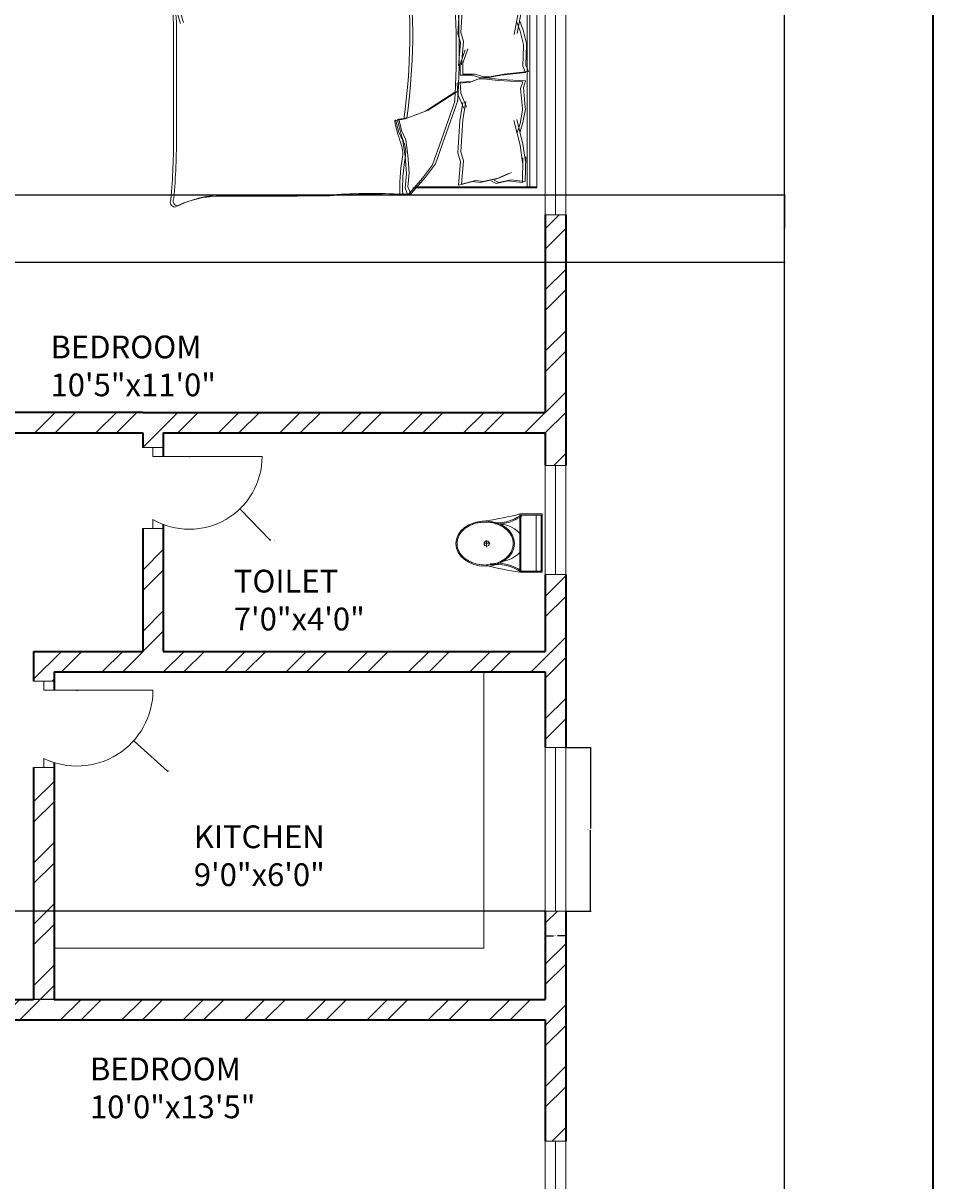
# Model space of a CAD drawing. Units: inches. Extents: x 2008 to 2657, y 1077 to 2165.
# Tile 7 of 16: x 2457 to 2657, y 1312 to 1567. Entities that reach past the tile are written whole.
import ezdxf

# ---------------------------------------------------------------- set-up
doc = ezdxf.new("R2010")
doc.units = ezdxf.units.IN
for name, color, linetype, lineweight in [('A-ANNO-DIMS', 2, 'Continuous', 18), ('A-ANNO-TTLB', 7, 'Continuous', 35), ('A-AREA-IDEN', 4, 'Continuous', 18), ('A-DOOR', 11, 'Continuous', 18), ('A-FLOR-CASE', 9, 'Continuous', 18), ('A-FLOR-FIXT', 8, 'Continuous', 18), ('A-FURN', 8, 'Continuous', 13), ('A-GLAZ', 191, 'Continuous', 18), ('A-WALL', 7, 'Continuous', 35)]:
    doc.layers.add(name, color=color, linetype=linetype, lineweight=lineweight)
doc.layers.add('A-WALL-PATT', color=30, linetype='Continuous', lineweight=13, true_color=0xf8991e)
doc.styles.get("Standard").update_dxf_attribs({"font": 'arial.ttf'})
doc.dimstyles.get("Standard").update_dxf_attribs({"dimtxt": 0.18, "dimasz": 0.18, "dimexe": 0.18, "dimexo": 0.0625, "dimgap": 0.09, "dimtad": 0, "dimtih": 1, "dimtoh": 1, "dimdec": 4, "dimzin": 0, "dimdsep": 46, "dimtxsty": 'Standard', "dimcen": 0.09, "dimadec": 0, "dimazin": 0, "dimtfac": 1, "dimtdec": 4, "dimtofl": 0, "dimtmove": 0, "dimatfit": 3, "dimfxl": 1, "dimtolj": 1, "dimtzin": 0, "dimarcsym": 0})

# ---------------------------------------------------------------- blocks, each defined once
blk = doc.blocks.new('A$C31115884')
for p, q in [((258, 466), (258, 523)), ((283, 498), (223, 498)), ((0, 200), (0, 0)), ((520, 200), (0, 200)), ((10, 190), (10, 10)), ((510, 190), (10, 190)), ((510, 10), (510, 190)), ((520, 0), (520, 200)), ((510, 54), (0, 54)), ((10, 10), (510, 10)), ((0, 0), (520, 0))]:
    blk.add_line(p, q)
blk.add_circle((256, 496), 23.6)
for centre, radius, start, end in [((2778, -205), 2807, 165.4549, 171.7133), ((-295, 403), 365, 324.2091, 9.3499), ((-295, 403), 375, 324.2091, 9.3499), ((139, 406), 293, 315.8436, 2.6563), ((806, 403), 365, 170.6501, 215.7909), ((3237, 905), 2807, 188.2867, 194.5451), ((384, 406), 293, 190.2774, 224.1564), ((806, 403), 375, 179.2036, 215.7909)]:
    blk.add_arc(centre, radius, start, end)
blk.add_ellipse((256, 510), major_axis=(0, -261), ratio=0.772727)
blk.add_open_spline([(256, 259), (263, 259), (270, 260), (288, 262), (299, 265), (320, 273), (330, 278), (350, 291), (360, 299), (378, 316), (386, 326), (402, 347), (409, 358), (421, 383), (427, 395), (436, 422), (440, 436), (445, 465), (447, 480), (448, 509), (448, 524), (445, 553), (443, 568), (436, 596), (432, 610), (422, 636), (416, 649), (402, 672), (395, 683), (379, 703), (370, 712), (351, 728), (341, 735), (321, 746), (310, 751), (289, 757), (278, 759), (256, 761), (245, 761), (223, 757), (212, 754), (191, 746), (181, 741), (161, 728), (151, 720), (133, 703), (125, 693), (110, 672), (103, 660), (90, 636), (85, 623), (76, 596), (72, 582), (67, 553), (66, 538), (64, 509), (65, 494), (68, 465), (70, 450), (77, 422), (81, 408), (91, 382), (97, 370), (111, 346), (118, 335), (135, 316), (144, 307), (162, 291), (172, 284), (193, 273), (203, 269), (225, 262), (236, 260), (250, 259), (253, 259), (256, 259)], degree=3, knots=[0, 0, 0, 0, 0.110105, 0.110105, 0.285049, 0.285049, 0.459994, 0.459994, 0.634938, 0.634938, 0.809882, 0.809882, 0.984827, 0.984827, 1.159771, 1.159771, 1.334715, 1.334715, 1.50966, 1.50966, 1.684604, 1.684604, 1.859549, 1.859549, 2.034493, 2.034493, 2.209437, 2.209437, 2.384382, 2.384382, 2.559326, 2.559326, 2.73427, 2.73427, 2.909215, 2.909215, 3.084159, 3.084159, 3.259103, 3.259103, 3.434048, 3.434048, 3.608992, 3.608992, 3.783936, 3.783936, 3.958881, 3.958881, 4.133825, 4.133825, 4.30877, 4.30877, 4.483714, 4.483714, 4.658658, 4.658658, 4.833603, 4.833603, 5.008547, 5.008547, 5.183491, 5.183491, 5.358436, 5.358436, 5.53338, 5.53338, 5.708324, 5.708324, 5.883269, 5.883269, 6.058213, 6.058213, 6.233158, 6.233158, 6.283185, 6.283185, 6.283185, 6.283185])
blk = doc.blocks.new('BED-DOUBLE')
for p, q in [((0, 51.49), (0.64, 51.49)), ((0, 3.48), (0, 51.49)), ((0, 51.27), (26.61, 51.27)), ((0, 51.27), (26.61, 51.27)), ((0.64, 51.49), (27.25, 51.49)), ((0.64, 51.49), (27.25, 51.49)), ((1.53, 3.48), (1.53, 51.27)), ((1.53, 3.48), (1.53, 51.27)), ((2.17, 3.7), (2.17, 51.49)), ((2.17, 3.7), (2.17, 51.49)), ((17.21, 50.93), (14.07, 50.15)), ((17.21, 50.93), (14.07, 50.15)), ((16.81, 45.8), (17.21, 50.93)), ((16.81, 45.8), (17.21, 50.93)), ((27.75, 52.87), (24.5, 49.16)), ((27.75, 52.87), (24.5, 49.16)), ((28.39, 53.1), (25.14, 49.39)), ((28.39, 53.1), (25.14, 49.39)), ((29.49, 52.95), (27.75, 52.87, 3.87)), ((29.49, 52.95), (27.75, 52.87, 3.87)), ((28.37, 51.33), (27.75, 52.87)), ((28.37, 51.33), (27.75, 52.87)), ((28.06, 48.23), (28.37, 51.33)), ((28.06, 48.23), (28.37, 51.33)), ((30.13, 53.18), (28.39, 53.1, 3.87)), ((30.13, 53.18), (28.39, 53.1, 3.87)), ((29, 51.56), (28.39, 53.1)), ((29, 51.56), (28.39, 53.1)), ((28.7, 48.46), (29, 51.56)), ((28.7, 48.46), (29, 51.56)), ((2.56, 50.11), (2.46, 44.71)), ((2.56, 50.11), (2.46, 44.71)), ((2.56, 50.11), (5.77, 49.73)), ((2.56, 50.11), (5.77, 49.73)), ((3.2, 50.34), (3.1, 44.94)), ((3.2, 50.34), (3.1, 44.94)), ((3.2, 50.34), (6.41, 49.96)), ((3.2, 50.34), (6.41, 49.96)), ((8.26, 49.31), (5.58, 48.13)), ((8.26, 49.31), (5.58, 48.13)), ((5.77, 49.73), (8.34, 50.33)), ((5.77, 49.73), (8.34, 50.33)), ((8.9, 49.54), (6.22, 48.36)), ((8.9, 49.54), (6.22, 48.36)), ((6.41, 49.96), (8.98, 50.56)), ((6.41, 49.96), (8.98, 50.56)), ((11.83, 50.11), (8.26, 49.31)), ((11.83, 50.11), (8.26, 49.31)), ((8.34, 50.33), (9.38, 49.82)), ((8.34, 50.33), (9.38, 49.81)), ((12.47, 50.34), (8.9, 49.54)), ((12.47, 50.34), (8.9, 49.54)), ((8.98, 50.56), (10.02, 50.04)), ((8.98, 50.56), (10.02, 50.04)), ((13.43, 49.92), (11.83, 50.11)), ((13.43, 49.92), (11.83, 50.11)), ((14.07, 50.15), (12.47, 50.34)), ((14.07, 50.15), (12.47, 50.34)), ((16.57, 50.7), (13.43, 49.92)), ((16.57, 50.7), (13.43, 49.92)), ((16.17, 45.57), (16.57, 50.7)), ((16.17, 45.57), (16.57, 50.7)), ((24.5, 49.16), (22.33, 46.22)), ((24.5, 49.16), (22.33, 46.22)), ((25.14, 49.39), (22.97, 46.45)), ((25.14, 49.39), (22.97, 46.45)), ((29, 44.59), (28.7, 48.46)), ((29, 44.59), (28.7, 48.46)), ((3.1, 44.94), (3.18, 45.94)), ((3.1, 44.94), (3.18, 45.94)), ((3.18, 45.94), (3.71, 42.14)), ((3.18, 45.94), (3.71, 42.14)), ((22.33, 46.22), (20.32, 40.64)), ((22.33, 46.22), (20.32, 40.64)), ((22.97, 46.45), (20.96, 40.87)), ((22.97, 46.45), (20.96, 40.87)), ((28.37, 44.36), (28.06, 48.23)), ((28.37, 44.36), (28.06, 48.23)), ((2.46, 44.71), (2.54, 45.71)), ((2.46, 44.71), (2.54, 45.71)), ((2.54, 45.71), (3.07, 41.91)), ((2.54, 45.71), (3.07, 41.91)), ((16.73, 43.61), (16.17, 45.57)), ((16.73, 43.61), (16.17, 45.57)), ((16.3, 36.6), (16.73, 43.61)), ((16.3, 36.6), (16.73, 43.61)), ((17.37, 43.84), (16.81, 45.8)), ((17.37, 43.83), (16.81, 45.8)), ((16.93, 36.83), (17.37, 43.84)), ((16.93, 36.82), (17.37, 43.83)), ((28.83, 40.95), (28.37, 44.36)), ((28.83, 40.95), (28.37, 44.36)), ((29.47, 41.18), (29, 44.59)), ((29.47, 41.18), (29, 44.59)), ((3.07, 41.91), (4.42, 36.5)), ((3.07, 41.91), (4.42, 36.5)), ((3.71, 42.14), (5.06, 36.72)), ((3.71, 42.14), (5.06, 36.72)), ((20.96, 40.87), (18.02, 32.54)), ((20.96, 40.87), (18.02, 32.53)), ((29.76, 38.94), (28.83, 40.95)), ((29.76, 38.94), (28.83, 40.95)), ((30.4, 39.17), (29.47, 41.18)), ((30.4, 39.17), (29.47, 41.18)), ((3.67, 39.2), (3.08, 37.14)), ((3.67, 39.2), (3.08, 37.14)), ((4.31, 39.43), (3.72, 37.36)), ((4.31, 39.43), (3.72, 37.36)), ((20.32, 40.64), (17.38, 32.31)), ((20.32, 40.64), (17.38, 32.31)), ((30.38, 36.46), (29.76, 38.94)), ((30.38, 36.46), (29.76, 38.94)), ((31.02, 36.69), (30.4, 39.17)), ((31.02, 36.69), (30.4, 39.17)), ((79.25, 15.06), (79.25, 39.68)), ((79.25, 15.06), (79.25, 39.68)), ((79.88, 15.29), (79.88, 39.91)), ((79.88, 15.29), (79.88, 39.91)), ((3.08, 37.14), (2.54, 34.21)), ((3.08, 37.14), (2.54, 34.2)), ((3.72, 37.36), (3.18, 34.43)), ((3.72, 37.36), (3.18, 34.43)), ((15.63, 32.56), (16.3, 36.6)), ((15.63, 32.56), (16.3, 36.6)), ((16.27, 32.79), (16.93, 36.83)), ((16.27, 32.79), (16.93, 36.82)), ((23.88, 34.45), (28.37, 36.15)), ((23.88, 34.45), (28.37, 36.15)), ((24.52, 34.68), (29, 36.38)), ((24.52, 34.68), (29, 36.38)), ((28.37, 36.15), (30.38, 36.46)), ((28.37, 36.15), (30.38, 36.46)), ((29, 36.38), (31.02, 36.69)), ((29, 36.38), (31.02, 36.69)), ((2.54, 34.21), (2.56, 33.88)), ((2.54, 34.2), (2.56, 33.88)), ((2.56, 33.88), (2.98, 29.46)), ((2.56, 33.88), (2.98, 29.46)), ((3.18, 34.43), (3.2, 34.11)), ((3.18, 34.43), (3.2, 34.11)), ((3.2, 34.11), (3.62, 29.68)), ((3.2, 34.11), (3.62, 29.68)), ((16.74, 30.75), (15.45, 33.82)), ((16.74, 30.75), (15.45, 33.82)), ((17.38, 30.98), (16.09, 34.05)), ((17.38, 30.98), (16.09, 34.05)), ((17.38, 30.26), (23.88, 34.45)), ((17.38, 30.26), (23.88, 34.45)), ((18.02, 30.49), (24.52, 34.68)), ((18.02, 30.49), (24.52, 34.68)), ((16.89, 28.3), (16.74, 30.75)), ((16.89, 28.3), (16.74, 30.75)), ((17.53, 28.53), (17.38, 30.98)), ((17.53, 28.53), (17.38, 30.98)), ((2.98, 29.46), (2.49, 27.98)), ((2.98, 29.46), (2.49, 27.98)), ((3.62, 29.68), (3.13, 28.21)), ((3.62, 29.68), (3.13, 28.21)), ((3.13, 28.21), (8.51, 27.96)), ((3.13, 28.21), (8.51, 27.96)), ((12.38, 27.44), (14.22, 28.13)), ((12.38, 27.44), (14.22, 28.13)), ((13.02, 27.66), (14.86, 28.36)), ((13.02, 27.66), (14.86, 28.36)), ((14.22, 28.13), (16.89, 28.3)), ((14.22, 28.13), (16.89, 28.3)), ((14.86, 28.36), (17.53, 28.53)), ((14.86, 28.36), (17.53, 28.53)), ((1.87, 25.98), (7.22, 26.56)), ((1.87, 25.98), (7.22, 26.56)), ((2.45, 24.54), (1.87, 25.98)), ((2.45, 24.54), (1.87, 25.98)), ((2.49, 27.98), (7.87, 27.73)), ((2.49, 27.98), (7.87, 27.73)), ((2.51, 26.21), (7.86, 26.79)), ((2.51, 26.21), (7.86, 26.79)), ((3.09, 24.77), (2.51, 26.21)), ((3.09, 24.77), (2.51, 26.21)), ((7.22, 26.56), (10.4, 27.14)), ((7.22, 26.56), (10.4, 27.14)), ((7.86, 26.79), (11.04, 27.37)), ((7.86, 26.79), (11.04, 27.37)), ((7.87, 27.73), (11.08, 27.36)), ((7.87, 27.73), (11.08, 27.36)), ((8.51, 27.96), (11.72, 27.58)), ((8.51, 27.96), (11.72, 27.58)), ((10.4, 27.14), (11.7, 27.14)), ((10.4, 27.14), (11.7, 27.14)), ((11.04, 27.37), (12.34, 27.37)), ((11.04, 27.37), (12.34, 27.37)), ((11.08, 27.36), (12.38, 27.44)), ((11.08, 27.36), (12.38, 27.44)), ((11.7, 27.14), (13.58, 26.56)), ((11.7, 27.14), (13.58, 26.56)), ((11.72, 27.58), (13.02, 27.66)), ((11.72, 27.58), (13.02, 27.66)), ((12.34, 27.37), (14.22, 26.79)), ((12.34, 27.37), (14.22, 26.79)), ((13.58, 26.56), (16.26, 26.56)), ((13.58, 26.56), (16.26, 26.56)), ((14.22, 26.79), (16.9, 26.79)), ((14.22, 26.79), (16.9, 26.79)), ((16.26, 26.56), (16.26, 24.1)), ((16.26, 26.56), (16.26, 24.1)), ((16.9, 26.79), (16.9, 24.33)), ((16.9, 26.79), (16.9, 24.33)), ((2.3, 20.09), (2.45, 24.54)), ((2.3, 20.09), (2.45, 24.54)), ((2.94, 20.32), (3.09, 24.77)), ((2.94, 20.32), (3.09, 24.77)), ((16.26, 24.1), (15.17, 20.96)), ((16.26, 24.1), (15.17, 20.96)), ((16.9, 24.33), (15.81, 21.19)), ((16.9, 24.33), (15.81, 21.19)), ((16.17, 19.38), (16.57, 24.52)), ((16.17, 19.38), (16.57, 24.52)), ((16.81, 19.61), (17.21, 24.74)), ((16.81, 19.61), (17.21, 24.74)), ((2.3, 19.77), (2.3, 20.09)), ((2.3, 19.77), (2.3, 20.09)), ((3.03, 16.88), (2.3, 19.77)), ((3.03, 16.88), (2.3, 19.77)), ((2.94, 20), (2.94, 20.32)), ((2.94, 20), (2.94, 20.32)), ((3.67, 17.11), (2.94, 20)), ((3.67, 17.11), (2.94, 20)), ((3.96, 12.34), (4.97, 17.83)), ((3.96, 12.34), (4.97, 17.83)), ((16.73, 17.42), (16.17, 19.38)), ((16.73, 17.42), (16.17, 19.38)), ((17.37, 17.65), (16.81, 19.61)), ((17.37, 17.65), (16.81, 19.61)), ((3.75, 14.86), (3.03, 16.88)), ((3.75, 14.86), (3.03, 16.88)), ((3.32, 12.11), (4.33, 17.6)), ((3.32, 12.11), (4.33, 17.6)), ((4.39, 15.08), (3.67, 17.11)), ((4.39, 15.08), (3.67, 17.11)), ((16.3, 10.41), (16.73, 17.42)), ((16.3, 10.41), (16.73, 17.42)), ((16.93, 10.64), (17.37, 17.65)), ((16.93, 10.64), (17.37, 17.65)), ((3.03, 8.29), (3.32, 12.11)), ((3.03, 8.29), (3.32, 12.11)), ((3.67, 8.51), (3.96, 12.34)), ((3.67, 8.51), (3.96, 12.34)), ((15.63, 6.38), (16.3, 10.41)), ((15.63, 6.38), (16.3, 10.41)), ((16.27, 6.61), (16.93, 10.64)), ((16.27, 6.61), (16.93, 10.64)), ((16.3, 10.41), (16.62, 9.28)), ((16.3, 10.41), (16.62, 9.28)), ((16.93, 10.64), (17.26, 9.51)), ((16.93, 10.64), (17.26, 9.51)), ((3.01, 8.18), (3.03, 8.29)), ((3.01, 8.18), (3.03, 8.29)), ((3.34, 3.9), (3.01, 8.18)), ((3.34, 3.9), (3.01, 8.18)), ((3.65, 8.41), (3.67, 8.51)), ((3.65, 8.41), (3.67, 8.51)), ((3.98, 4.13), (3.65, 8.41)), ((3.98, 4.13), (3.65, 8.41)), ((16.62, 9.28), (17.34, 4.18)), ((16.62, 9.28), (17.34, 4.18)), ((17.26, 9.51), (17.98, 4.41)), ((17.26, 9.51), (17.98, 4.41)), ((8.96, 5.05), (6.21, 6.06)), ((8.96, 5.05), (6.21, 6.06)), ((9.59, 5.28), (6.85, 6.29)), ((9.59, 5.28), (6.85, 6.29)), ((13.21, 4.7), (9.59, 5.28)), ((13.21, 4.7), (9.59, 5.28)), ((18.11, 3.48), (0, 3.48)), ((18.11, 3.48), (0, 3.48)), ((18.75, 3.7), (0.64, 3.7)), ((18.75, 3.7), (0.64, 3.7)), ((3.32, 3.9), (6.5, 4.47)), ((3.32, 3.89), (6.5, 4.47)), ((3.96, 4.12), (7.14, 4.7)), ((3.96, 4.12), (7.14, 4.7)), ((6.5, 4.47), (9.1, 4.04)), ((6.5, 4.47), (9.1, 4.04)), ((7.14, 4.7), (9.74, 4.27)), ((7.14, 4.7), (9.74, 4.27)), ((12.57, 4.47), (8.96, 5.05)), ((12.57, 4.47), (8.96, 5.05)), ((9.1, 4.04), (10.11, 4.62)), ((9.1, 4.04), (10.11, 4.62)), ((9.74, 4.27), (10.75, 4.85)), ((9.74, 4.27), (10.75, 4.85)), ((14.16, 4.76), (12.57, 4.47)), ((14.16, 4.76), (12.57, 4.47)), ((14.8, 4.99), (13.21, 4.7)), ((14.8, 4.99), (13.21, 4.7)), ((17.34, 4.18), (14.16, 4.76)), ((17.34, 4.18), (14.16, 4.76)), ((17.98, 4.41), (14.8, 4.99)), ((17.98, 4.41), (14.8, 4.99))]:
    blk.add_line(p, q)
for centre, radius, start, end in [((68.67, 76.16), 23.07, 267.4714, 296.4681), ((68.67, 76.16), 23.07, 267.4714, 296.4681), ((69.31, 76.39), 23.07, 267.4714, 296.4681), ((69.31, 76.39), 23.07, 267.4714, 296.4681), ((78.87, 54.41), 1.1, 332.6588, 86.02), ((78.87, 54.41), 1.1, 332.6588, 86.02), ((212.28, 41.15), 133.04, 174.4998, 180.6351), ((212.28, 41.15), 133.04, 174.4998, 180.6351), ((79.51, 54.64), 1.1, 332.6588, 86.02), ((79.51, 54.64), 1.1, 332.6588, 86.02), ((212.92, 41.38), 133.04, 174.4998, 180.6351), ((212.92, 41.38), 133.04, 174.4998, 180.6351), ((-6.66, 51.33), 36.18, 349.8763, 2.5657), ((-6.66, 51.33), 36.18, 349.8763, 2.5657), ((36.32, 182.27), 129.5, 266.9791, 273.8365), ((36.32, 182.27), 129.5, 266.9791, 273.8365), ((-6.02, 51.56), 36.18, 349.8763, 2.5657), ((-6.02, 51.56), 36.18, 349.8763, 2.5657), ((36.95, 182.49), 129.5, 266.9791, 273.8365), ((36.95, 182.49), 129.5, 266.9791, 273.8365), ((67.82, -4508.74), 4561.86, 90.00217, 90.28689), ((67.82, -4508.74), 4561.86, 90.00217, 90.28689), ((68.46, -4508.51), 4561.86, 90.00217, 90.28689), ((68.46, -4508.51), 4561.86, 90.00217, 90.28689), ((35.07, 43.74), 6.22, 168.6608, 203.7384), ((35.07, 43.74), 6.22, 168.6608, 203.7384), ((35.71, 43.97), 6.22, 168.6608, 203.7384), ((35.71, 43.97), 6.22, 168.6608, 203.7384), ((1.48, 31.15), 29.65, 10.6617, 19.8806), ((1.48, 31.15), 29.65, 10.6617, 19.8806), ((2.12, 31.38), 29.65, 10.6617, 19.8806), ((2.12, 31.38), 29.65, 10.6617, 19.8806), ((156.32, 17.76), 129.02, 171.7845, 186.9006), ((156.32, 17.76), 129.02, 171.7845, 186.9006), ((156.96, 17.98), 129.02, 171.7845, 186.9006), ((156.96, 17.98), 129.02, 171.7845, 186.9006), ((30.44, 36.64), 0.185, 250.2464, 1.1377), ((30.44, 36.64), 0.185, 250.2464, 1.1377), ((31.08, 36.87), 0.185, 250.2464, 1.1377), ((31.08, 36.86), 0.185, 250.2464, 1.1377), ((182.05, 21.36), 164.97, 176.0865, 186.7821), ((182.05, 21.36), 164.97, 176.0865, 186.7821), ((182.69, 21.59), 164.97, 176.0865, 186.7821), ((182.69, 21.59), 164.97, 176.0865, 186.7821), ((-23.07, -16.99), 106.46, 13.3832, 17.7053), ((-23.07, -16.99), 106.46, 13.3832, 17.7053), ((201.48, 21.66), 121.76, 182.9958, 189.4091), ((201.48, 21.66), 121.76, 182.9958, 189.4091), ((-23.71, -17.22), 106.46, 13.3832, 17.7053), ((-23.71, -17.22), 106.46, 13.3832, 17.7053), ((200.84, 21.43), 121.76, 182.9958, 189.4091), ((200.84, 21.43), 121.76, 182.9958, 189.4091), ((31.17, -167.31), 170.11, 88.4762, 91.0082), ((31.17, -167.31), 170.11, 88.4762, 91.0082), ((31.81, -167.08), 170.11, 88.4762, 91.0082), ((31.81, -167.08), 170.11, 88.4762, 91.0082), ((50.61, 484.82), 482.31, 268.2277, 271.7185), ((50.61, 484.82), 482.31, 268.2277, 271.7185), ((51.25, 485.05), 482.31, 268.2277, 271.7185), ((51.25, 485.05), 482.31, 268.2277, 271.7185), ((64.52, -26.9), 29.63, 76.0648, 88.9113), ((64.52, -26.9), 29.63, 76.0648, 88.9113), ((65.15, -26.67), 29.63, 76.0648, 88.9113), ((65.15, -26.67), 29.63, 76.0648, 88.9113), ((20.1, 85.16), 83.31, 268.7218, 275.604), ((20.1, 85.16), 83.31, 268.7218, 275.604), ((20.74, 85.39), 83.31, 268.7218, 275.604), ((20.74, 85.39), 83.31, 268.7218, 275.604), ((70.28, -21.66), 23.56, 67.9751, 86.652), ((70.28, -21.66), 23.56, 67.9751, 86.652), ((70.92, -21.43), 23.56, 67.9751, 86.652), ((70.92, -21.43), 23.56, 67.9751, 86.652), ((79.72, 1.09), 1.09, 236.1736, 23.4781), ((79.72, 1.09), 1.09, 236.1736, 23.4781), ((80.36, 1.32), 1.09, 236.1736, 23.4781), ((80.36, 1.32), 1.09, 236.1736, 23.4781)]:
    blk.add_arc(centre, radius, start, end)
blk = doc.blocks.new('WIN-60IN-B')
for p, q in [((0, 4.5), (0, 0)), ((0, 4.5), (60, 4.5)), ((60, 2.25), (60, 4.5)), ((60, 4.5), (60, 0)), ((0, 0), (0, 2.25)), ((0, 2.25), (60, 2.25)), ((60, 0), (0, 0))]:
    blk.add_line(p, q)
blk = doc.blocks.new('WIN-24IN-B')
for p, q in [((0, 24), (4.5, 24)), ((0, 24), (0, 0)), ((4.5, 24), (2.25, 24)), ((2.25, 24), (2.25, 0)), ((4.5, 0), (4.5, 24)), ((2.25, 0), (0, 0)), ((0, 0), (4.5, 0))]:
    blk.add_line(p, q)
blk = doc.blocks.new('WIN-36IN-A')
for p, q in [((0, 36), (4.5, 36)), ((0, 0), (0, 36)), ((4.5, 36), (2.25, 36)), ((2.25, 36), (2.25, 0)), ((4.5, 36), (4.5, 0)), ((4.5, 0), (0, 0)), ((2.25, 0), (4.5, 0))]:
    blk.add_line(p, q)
blk = doc.blocks.new('*D27')
at = {"layer": 'A-ANNO-DIMS', "color": 0, "lineweight": -2, "transparency": 16777216}
for p, q in [((2576.82, 1407.57), (2582.34, 1407.57)), ((2582.16, 1407.39), (2582.16, 1389.75)), ((2582.16, 1371.75), (2582.16, 1389.39)), ((2576.82, 1371.57), (2582.34, 1371.57))]:
    blk.add_line(p, q, dxfattribs=at)
at = {"layer": 'A-ANNO-DIMS', "color": 0, "transparency": 16777216}
for points in [[(2582.13, 1407.39), (2582.19, 1407.39), (2582.16, 1407.57)], [(2582.13, 1371.75), (2582.19, 1371.75), (2582.16, 1371.57)]]:
    blk.add_solid(points, dxfattribs=at)
at = {"layer": 'Defpoints', "color": 0, "transparency": 16777216}
for p in [(2576.76, 1407.57), (2582.16, 1407.57), (2576.76, 1371.57)]:
    blk.add_point(p, dxfattribs=at)
at = {"layer": 'A-ANNO-DIMS', "color": 0, "transparency": 16777216, "insert": (2582.16, 1389.57), "char_height": 0.18, "attachment_point": 5}
blk.add_mtext('\\A1;WIN A 36 TYP.', dxfattribs=at)
blk = doc.blocks.new('*D28')
at = {"layer": 'A-ANNO-DIMS', "color": 0, "lineweight": -2, "transparency": 16777216}
for p, q in [((2572.26, 1371.51), (2572.26, 1365.99)), ((2576.76, 1371.51), (2576.76, 1365.99)), ((2572.44, 1366.17), (2574.05, 1366.17)), ((2576.58, 1366.17), (2574.97, 1366.17))]:
    blk.add_line(p, q, dxfattribs=at)
at = {"layer": 'A-ANNO-DIMS', "color": 0, "transparency": 16777216}
for points in [[(2572.44, 1366.2), (2572.44, 1366.14), (2572.26, 1366.17)], [(2576.58, 1366.2), (2576.58, 1366.14), (2576.76, 1366.17)]]:
    blk.add_solid(points, dxfattribs=at)
at = {"layer": 'Defpoints', "color": 0, "transparency": 16777216}
for p in [(2572.26, 1371.57), (2576.76, 1371.57), (2576.76, 1366.17)]:
    blk.add_point(p, dxfattribs=at)
at = {"layer": 'A-ANNO-DIMS', "color": 0, "transparency": 16777216, "insert": (2574.51, 1366.17), "char_height": 0.18, "attachment_point": 5}
blk.add_mtext('\\A1;5 TYP.', dxfattribs=at)
blk = doc.blocks.new('*D31')
at = {"layer": 'A-ANNO-DIMS', "color": 0, "lineweight": -2, "transparency": 16777216}
for p, q in [((2076.26, 1562.18), (2076.26, 1140.44)), ((2576.76, 1188.61), (2576.76, 1140.44)), ((2076.44, 1140.62), (2326.12, 1140.62)), ((2576.58, 1140.62), (2326.91, 1140.62))]:
    blk.add_line(p, q, dxfattribs=at)
at = {"layer": 'A-ANNO-DIMS', "color": 0, "transparency": 16777216}
for points in [[(2076.44, 1140.65), (2076.44, 1140.59), (2076.26, 1140.62)], [(2576.58, 1140.65), (2576.58, 1140.59), (2576.76, 1140.62)]]:
    blk.add_solid(points, dxfattribs=at)
at = {"layer": 'Defpoints', "color": 0, "transparency": 16777216}
for p in [(2076.26, 1562.24), (2576.76, 1188.67), (2576.76, 1140.62)]:
    blk.add_point(p, dxfattribs=at)
at = {"layer": 'A-ANNO-DIMS', "color": 0, "transparency": 16777216, "insert": (2326.51, 1140.62), "char_height": 0.18, "attachment_point": 5}
blk.add_mtext('\\A1;500.5', dxfattribs=at)
blk = doc.blocks.new('*D32')
at = {"layer": 'A-ANNO-DIMS', "color": 0, "lineweight": -2, "transparency": 16777216}
for p, q in [((2576.82, 2094.67), (2624.99, 2094.67)), ((2624.81, 2094.49), (2624.81, 1641.86)), ((2624.81, 1188.85), (2624.81, 1641.49)), ((2576.82, 1188.67), (2624.99, 1188.67))]:
    blk.add_line(p, q, dxfattribs=at)
at = {"layer": 'A-ANNO-DIMS', "color": 0, "transparency": 16777216}
for points in [[(2624.78, 2094.49), (2624.84, 2094.49), (2624.81, 2094.67)], [(2624.78, 1188.85), (2624.84, 1188.85), (2624.81, 1188.67)]]:
    blk.add_solid(points, dxfattribs=at)
at = {"layer": 'Defpoints', "color": 0, "transparency": 16777216}
for p in [(2576.76, 2094.67), (2624.81, 2094.67), (2576.76, 1188.67)]:
    blk.add_point(p, dxfattribs=at)
at = {"layer": 'A-ANNO-DIMS', "color": 0, "transparency": 16777216, "insert": (2624.81, 1641.67), "char_height": 0.18, "attachment_point": 5}
blk.add_mtext('\\A1;906', dxfattribs=at)
blk = doc.blocks.new('*D68')
at = {"layer": 'A-ANNO-DIMS', "color": 0, "lineweight": -2, "transparency": 16777216}
for p, q in [((2572.2, 1371.57), (2028.03, 1371.57)), ((2028.21, 1371.39), (2028.21, 1362.05)), ((2028.21, 1352.35), (2028.21, 1361.69)), ((2572.2, 1352.17), (2028.03, 1352.17))]:
    blk.add_line(p, q, dxfattribs=at)
at = {"layer": 'A-ANNO-DIMS', "color": 0, "transparency": 16777216}
for points in [[(2028.18, 1371.39), (2028.24, 1371.39), (2028.21, 1371.57)], [(2028.18, 1352.35), (2028.24, 1352.35), (2028.21, 1352.17)]]:
    blk.add_solid(points, dxfattribs=at)
at = {"layer": 'Defpoints', "color": 0, "transparency": 16777216}
for p in [(2028.21, 1371.57), (2572.26, 1371.57), (2572.26, 1352.17)]:
    blk.add_point(p, dxfattribs=at)
at = {"layer": 'A-ANNO-DIMS', "color": 0, "transparency": 16777216, "insert": (2028.21, 1361.87), "char_height": 0.18, "attachment_point": 5}
blk.add_mtext('\\A1;19.394', dxfattribs=at)
blk = doc.blocks.new('*D69')
at = {"layer": 'A-ANNO-DIMS', "color": 0, "lineweight": -2, "transparency": 16777216}
for p, q in [((2109.32, 1529), (2624.99, 1529)), ((2624.81, 1528.82), (2624.81, 1521.8)), ((2624.81, 1514.42), (2624.81, 1521.44)), ((2109.32, 1514.24), (2624.99, 1514.24))]:
    blk.add_line(p, q, dxfattribs=at)
at = {"layer": 'A-ANNO-DIMS', "color": 0, "transparency": 16777216}
for points in [[(2624.78, 1528.82), (2624.84, 1528.82), (2624.81, 1529)], [(2624.78, 1514.42), (2624.84, 1514.42), (2624.81, 1514.24)]]:
    blk.add_solid(points, dxfattribs=at)
at = {"layer": 'Defpoints', "color": 0, "transparency": 16777216}
for p in [(2109.26, 1529), (2624.81, 1529), (2109.26, 1514.24)]:
    blk.add_point(p, dxfattribs=at)
at = {"layer": 'A-ANNO-DIMS', "color": 0, "transparency": 16777216, "insert": (2624.81, 1521.62), "char_height": 0.18, "attachment_point": 5}
blk.add_mtext('\\A1;14.756', dxfattribs=at)
blk = doc.blocks.new('*D94')
at = {"layer": 'A-ANNO-DIMS', "color": 0, "lineweight": -2, "transparency": 16777216}
for p, q in [((2493.94, 1471.51), (2494.12, 1471.51)), ((2494.03, 1471.42), (2494.03, 1471.6)), ((2511.77, 1453.08), (2505.24, 1459.86)), ((2511.95, 1453.08), (2511.77, 1453.08))]:
    blk.add_line(p, q, dxfattribs=at)
at = {"layer": 'A-ANNO-DIMS', "color": 0, "transparency": 16777216}
blk.add_solid([(2505.26, 1459.88), (2505.22, 1459.84), (2505.12, 1459.99)], dxfattribs=at)
at = {"layer": 'Defpoints', "color": 0, "transparency": 16777216}
for p in [(2494.03, 1471.51), (2505.12, 1459.99)]:
    blk.add_point(p, dxfattribs=at)
at = {"layer": 'A-ANNO-DIMS', "color": 0, "transparency": 16777216, "insert": (2512.5, 1453.08), "char_height": 0.18, "attachment_point": 5}
blk.add_mtext('\\A1;R15.985', dxfattribs=at)
blk = doc.blocks.new('*D95')
at = {"layer": 'A-ANNO-DIMS', "color": 0, "lineweight": -2, "transparency": 16777216}
for p, q in [((2469.23, 1420.15), (2469.41, 1420.15)), ((2469.32, 1420.06), (2469.32, 1420.24)), ((2489.24, 1402.36), (2481.9, 1408.91)), ((2489.42, 1402.36), (2489.24, 1402.36))]:
    blk.add_line(p, q, dxfattribs=at)
at = {"layer": 'A-ANNO-DIMS', "color": 0, "transparency": 16777216}
blk.add_solid([(2481.92, 1408.93), (2481.88, 1408.89), (2481.77, 1409.03)], dxfattribs=at)
at = {"layer": 'Defpoints', "color": 0, "transparency": 16777216}
for p in [(2469.32, 1420.15), (2481.77, 1409.03)]:
    blk.add_point(p, dxfattribs=at)
at = {"layer": 'A-ANNO-DIMS', "color": 0, "transparency": 16777216, "insert": (2489.97, 1402.36), "char_height": 0.18, "attachment_point": 5}
blk.add_mtext('\\A1;R16.696', dxfattribs=at)

msp = doc.modelspace()

# ---------------------------------------------------------------- hatches: boundary and pattern name
at = {"layer": 'A-WALL-PATT'}
h = msp.add_hatch(dxfattribs=at)
h.set_pattern_fill('ANSI32', color=256)
h.paths.add_polyline_path([(2109.2619, 2094.6743), (2104.7619, 2094.6743), (2104.7619, 2072.1743), (2104.7619, 2021.6151), (2109.2619, 2021.6151), (2109.2619, 2055.6743), (2126.1387, 2055.6743), (2126.1387, 2057.9243), (2126.1387, 2060.1743), (2109.2619, 2060.1743)])
h.paths.add_polyline_path([(2223.2494, 2057.9243), (2223.2494, 2060.1743), (2186.1387, 2060.1743), (2186.1387, 2055.6743), (2223.2494, 2055.6743)])
h.paths.add_polyline_path([(2250.7619, 2072.1743), (2250.7619, 2090.1743), (2250.7619, 2094.6743), (2246.2619, 2094.6743), (2246.2619, 2060.1743), (2242.7242, 2060.1743), (2242.7242, 2055.6743), (2246.2619, 2055.6743), (2246.2619, 1899.6743), (2242.7458, 1899.6743), (2242.7458, 1897.4243), (2242.7458, 1895.1743), (2246.2619, 1895.1743), (2246.2619, 1878.8745), (2248.5119, 1878.8745), (2250.7619, 1878.8745), (2250.7619, 1991.1743), (2250.7619, 2025.6743), (2257.6798, 2025.6743), (2257.6798, 2027.9243), (2257.6798, 2030.1743), (2250.7619, 2030.1743)])
h.paths.add_polyline_path([(2411.2619, 2031.6743), (2409.0119, 2031.6743), (2406.7619, 2031.6743), (2406.7619, 2030.1743), (2322.7619, 2030.1743), (2322.7619, 2053.3443), (2318.2619, 2053.3443), (2318.2619, 2030.1743), (2305.6798, 2030.1743), (2305.6798, 2025.6743), (2318.2619, 2025.6743), (2322.7619, 2025.6743), (2406.7619, 2025.6743), (2406.7619, 1995.6743), (2406.7619, 1847.2677), (2250.7619, 1847.2677), (2250.7619, 1850.9902), (2248.5119, 1850.9902), (2246.2619, 1850.9902), (2246.2619, 1847.1743), (2246.2619, 1842.7677), (2303.0015, 1842.7677), (2303.0015, 1667.2413), (2298.4208, 1667.2413), (2298.4208, 1662.7413), (2303.0015, 1662.7413), (2303.0015, 1649.8758), (2307.5015, 1649.8758), (2307.5015, 1842.7677), (2406.7619, 1842.7677), (2411.2619, 1842.7677), (2411.2619, 1878.6743), (2415.8196, 1878.6743), (2415.8196, 1880.9243), (2415.8196, 1883.1743), (2411.2619, 1883.1743)])
h.paths.add_polyline_path([(2411.2619, 2094.6743), (2406.7619, 2094.6743), (2318.2619, 2094.6743), (2318.2619, 2077.3443), (2322.7619, 2077.3443), (2322.7619, 2090.1743), (2406.7619, 2090.1743), (2406.7619, 2072.1743), (2406.7619, 2067.6743), (2406.7619, 2052.7524), (2411.2619, 2052.7524), (2411.2619, 2055.6743), (2414.9888, 2055.6743), (2414.9888, 2057.9243), (2414.9888, 2060.1743), (2411.2619, 2060.1743), (2411.2619, 2072.1743)])
h.paths.add_polyline_path([(2576.7619, 2072.1743), (2576.7619, 2094.6743), (2572.2619, 2094.6743), (2572.2619, 2060.1743), (2525.8113, 2060.1743), (2525.8113, 2055.6743), (2572.2619, 2055.6743), (2572.2619, 1994.289), (2576.7619, 1994.289)])
h.paths.add_polyline_path([(2465.8113, 2060.1743), (2436.2802, 2060.1743), (2436.2802, 2055.6743), (2465.8113, 2055.6743), (2465.8113, 2057.9243)])
h.paths.add_polyline_path([(2576.7619, 1934.289), (2574.5119, 1934.289), (2572.2619, 1934.289), (2572.2619, 1883.1743), (2447.7027, 1883.1743), (2447.7027, 1878.6743), (2459.7619, 1878.6743), (2459.7619, 1830.4982), (2464.2619, 1830.4982), (2464.2619, 1878.6743), (2572.2619, 1878.6743), (2572.2619, 1868.4883), (2576.7619, 1868.4883)])
h.paths.add_polyline_path([(2576.7619, 1832.4883), (2572.2619, 1832.4883), (2572.2619, 1806.6743), (2464.2619, 1806.6743), (2464.2619, 1809.6629), (2459.7619, 1809.6629), (2459.7619, 1802.1743), (2483.7619, 1802.1743), (2483.7619, 1778.1743), (2488.2619, 1778.1743), (2488.2619, 1802.1743), (2572.2619, 1802.1743), (2572.2619, 1793.6101), (2576.7619, 1793.6101)])
h.paths.add_polyline_path([(2576.7619, 1769.6101), (2572.2619, 1769.6101), (2572.2619, 1754.1743), (2488.2619, 1754.1743), (2488.2619, 1757.2675), (2486.0119, 1757.2675), (2483.7619, 1757.2675), (2483.7619, 1754.1743), (2447.4528, 1754.1743), (2447.4528, 1749.6743), (2483.7619, 1749.6743), (2572.2619, 1749.6743), (2572.2619, 1715.1837), (2576.7619, 1715.1837)])
h.paths.add_polyline_path([(2576.7619, 1655.1837), (2572.2619, 1655.1837), (2572.2619, 1617.6743), (2411.2619, 1617.6743), (2411.2619, 1749.6743), (2414.2827, 1749.6743), (2414.2827, 1754.1743), (2406.7619, 1754.1743), (2406.7619, 1749.6743), (2406.7619, 1617.6743), (2307.5015, 1617.6743), (2307.5015, 1621.0007), (2305.2515, 1621.0007), (2303.0015, 1621.0007), (2303.0015, 1609.6944), (2307.5015, 1609.6944), (2307.5015, 1613.1743), (2406.7619, 1613.1743), (2406.7619, 1476.6743), (2415.532, 1476.6743), (2415.532, 1478.9243), (2415.532, 1481.1743), (2411.2619, 1481.1743), (2411.2619, 1613.1743), (2572.2619, 1613.1743), (2572.2619, 1584.6086), (2576.7619, 1584.6086)])
h.paths.add_polyline_path([(2576.7619, 1524.6086), (2572.2619, 1524.6086), (2572.2619, 1481.1743), (2483.7619, 1481.1743), (2447.5119, 1481.1743), (2447.5119, 1476.6743), (2483.7619, 1476.6743), (2483.7619, 1473.5051), (2488.2619, 1473.5051), (2488.2619, 1476.6743), (2572.2619, 1476.6743), (2572.2619, 1469.5488), (2576.7619, 1469.5488)])
h.paths.add_polyline_path([(2576.7619, 1445.5488), (2572.2619, 1445.5488), (2572.2619, 1428.6743), (2488.2619, 1428.6743), (2488.2619, 1455.6743), (2486.0119, 1455.6743), (2483.7619, 1455.6743), (2483.7619, 1428.6743), (2459.7619, 1428.6743), (2459.7619, 1422.1519), (2464.2619, 1422.1519), (2464.2619, 1424.1743), (2572.2619, 1424.1743), (2572.2619, 1407.5685), (2576.7619, 1407.5685)])
h.paths.add_polyline_path([(2576.7619, 1371.5685), (2572.2619, 1371.5685), (2572.2619, 1352.1743), (2464.2619, 1352.1743), (2464.2619, 1403.1384), (2462.0119, 1403.1384), (2459.7619, 1403.1384), (2459.7619, 1352.1743), (2446.3194, 1352.1743), (2446.3194, 1347.6743), (2572.2619, 1347.6743), (2572.2619, 1321.0291), (2576.7619, 1321.0291)])
h.paths.add_polyline_path([(2462.703, 1227.6743), (2436.0298, 1227.6743), (2436.0298, 1225.4243), (2436.0298, 1223.1743), (2462.703, 1223.1743), (2462.703, 1225.4243)])
h.paths.add_polyline_path([(2576.7619, 1261.0291), (2574.5119, 1261.0291), (2572.2619, 1261.0291), (2572.2619, 1227.6743), (2522.703, 1227.6743), (2522.703, 1223.1743), (2572.2619, 1223.1743), (2572.2619, 1188.6743), (2576.7619, 1188.6743), (2576.7619, 1193.1743), (2576.7619, 1223.1743)])
h.paths.add_polyline_path([(2414.2823, 1227.6743), (2411.2619, 1227.6743), (2411.2619, 1267.1779), (2409.0119, 1267.1779), (2406.7619, 1267.1779), (2406.7619, 1227.6743), (2322.7619, 1227.6743), (2322.7619, 1244.3623), (2318.2619, 1244.3623), (2318.2619, 1223.1743), (2406.7619, 1223.1743), (2406.7619, 1193.1743), (2406.7619, 1188.6743), (2411.2619, 1188.6743), (2411.2619, 1193.1743), (2411.2619, 1223.1743), (2414.2823, 1223.1743)])
h.paths.add_polyline_path([(2411.2619, 1347.6743), (2414.702, 1347.6743), (2414.702, 1349.9243), (2414.702, 1352.1743), (2411.2619, 1352.1743), (2411.2619, 1416.7413), (2307.5015, 1416.7413), (2307.5015, 1579.8489), (2305.2515, 1579.8489), (2303.0015, 1579.8489), (2303.0015, 1566.7413), (2299.2719, 1566.7413), (2299.2719, 1562.2413), (2303.0015, 1562.2413), (2303.0015, 1416.7413), (2246.2619, 1416.7413), (2246.2619, 1409.8616), (2250.7619, 1409.8616), (2250.7619, 1412.2413), (2406.7619, 1412.2413), (2406.7619, 1292.1743), (2304.9703, 1292.1743), (2304.9703, 1287.6743), (2318.2619, 1287.6743), (2318.2619, 1268.3623), (2322.7619, 1268.3623), (2322.7619, 1287.6743), (2406.7619, 1287.6743), (2406.7619, 1285.4748), (2411.2619, 1285.4748)])
h.paths.add_polyline_path([(2109.2619, 1262.7482), (2104.7619, 1262.7482), (2104.7619, 1223.1743), (2104.7619, 1193.1743), (2104.7619, 1188.6743), (2109.2619, 1188.6743), (2109.2619, 1223.1743), (2126.7928, 1223.1743), (2126.7928, 1225.4243), (2126.7928, 1227.6743), (2109.2619, 1227.6743)])
h.paths.add_polyline_path([(2222.3268, 1227.6743), (2186.7928, 1227.6743), (2186.7928, 1223.1743), (2222.3268, 1223.1743)])
h.paths.add_polyline_path([(2250.7619, 1287.6743), (2256.9703, 1287.6743), (2256.9703, 1289.9243), (2256.9703, 1292.1743), (2250.7619, 1292.1743), (2250.7619, 1382.2078), (2248.5119, 1382.2078), (2246.2619, 1382.2078), (2246.2619, 1347.6743), (2246.2619, 1227.6743), (2242.6068, 1227.6743), (2242.6068, 1223.1743), (2246.2619, 1223.1743), (2246.2619, 1188.6743), (2250.7619, 1188.6743), (2250.7619, 1193.1743), (2250.7619, 1227.6743)])
h.paths.add_polyline_path([(2133.2619, 1349.9243), (2133.2619, 1352.1743), (2109.2619, 1352.1743), (2109.2619, 1375.2826), (2104.7619, 1375.2826), (2104.7619, 1322.7482), (2109.2619, 1322.7482), (2109.2619, 1347.6743), (2133.2619, 1347.6743)])
h.paths.add_polyline_path([(2210.2105, 1352.1743), (2161.7619, 1352.1743), (2161.7619, 1412.2413), (2185.7619, 1412.2413), (2185.7619, 1420.1851), (2183.5119, 1420.1851), (2181.2619, 1420.1851), (2181.2619, 1416.7413), (2109.2619, 1416.7413), (2109.2619, 1452.4006), (2104.7619, 1452.4006), (2104.7619, 1399.2826), (2109.2619, 1399.2826), (2109.2619, 1412.2413), (2157.2619, 1412.2413), (2157.2619, 1352.1743), (2154.3383, 1352.1743), (2154.3383, 1347.6743), (2210.2105, 1347.6743)])
h.paths.add_polyline_path([(2185.7619, 1514.2413), (2161.7619, 1514.2413), (2161.7619, 1518.1307), (2159.5119, 1518.1307), (2157.2619, 1518.1307), (2157.2619, 1514.2413), (2109.2619, 1514.2413), (2109.2619, 1528.997), (2107.0119, 1528.997), (2104.7619, 1528.997), (2104.7619, 1488.4006), (2109.2619, 1488.4006), (2109.2619, 1509.7413), (2181.2619, 1509.7413), (2181.2619, 1441.2042), (2185.7619, 1441.2042)])
h.paths.add_polyline_path([(2270.4025, 1566.7413), (2109.2619, 1566.7413), (2080.7619, 1566.7413), (2080.7619, 1586.5643), (2076.2619, 1586.5643), (2076.2619, 1562.2413), (2080.7619, 1562.2413), (2104.7619, 1562.2413), (2104.7619, 1552.997), (2109.2619, 1552.997), (2109.2619, 1562.2413), (2157.2619, 1562.2413), (2157.2619, 1538.2413), (2161.7619, 1538.2413), (2161.7619, 1562.2413), (2205.2619, 1562.2413), (2270.4025, 1562.2413)])
h.paths.add_polyline_path([(2131.6813, 1897.4243), (2131.6813, 1899.6743), (2109.2619, 1899.6743), (2109.2619, 1961.6151), (2104.7619, 1961.6151), (2104.7619, 1886.8042), (2109.2619, 1886.8042), (2109.2619, 1895.1743), (2131.6813, 1895.1743)])
h.paths.add_polyline_path([(2185.7619, 1847.1743), (2161.7619, 1847.1743), (2161.7619, 1895.1743), (2185.7619, 1895.1743), (2211.543, 1895.1743), (2211.543, 1897.4243), (2211.543, 1899.6743), (2154.0916, 1899.6743), (2154.0916, 1897.4243), (2154.0916, 1895.1743), (2157.2619, 1895.1743), (2157.2619, 1847.1743), (2109.2619, 1847.1743), (2109.2619, 1862.8042), (2104.7619, 1862.8042), (2104.7619, 1821.243), (2109.2619, 1821.243), (2109.2619, 1842.6743), (2181.2619, 1842.6743), (2181.2619, 1840.6763), (2185.7619, 1840.6763)])
h.paths.add_polyline_path([(2109.2619, 1785.243), (2104.7619, 1785.243), (2104.7619, 1715.4691), (2109.2619, 1715.4691), (2109.2619, 1730.8423), (2157.2619, 1730.8423), (2157.2619, 1727.6404), (2161.7619, 1727.6404), (2161.7619, 1730.8423), (2185.7619, 1730.8423), (2185.7619, 1822.1438), (2183.5119, 1822.1438), (2181.2619, 1822.1438), (2181.2619, 1735.3423), (2109.2619, 1735.3423)])
h.paths.add_polyline_path([(2109.2619, 1691.4691), (2104.7619, 1691.4691), (2104.7619, 1667.2413), (2076.2619, 1667.2413), (2076.2619, 1646.5643), (2080.7619, 1646.5643), (2080.7619, 1662.7413), (2109.2619, 1662.7413), (2271.4941, 1662.7413), (2271.4941, 1664.9913), (2271.4941, 1667.2413), (2181.2619, 1667.2413), (2161.7619, 1667.2413), (2161.7619, 1708.3752), (2159.5119, 1708.3752), (2157.2619, 1708.3752), (2157.2619, 1667.2413), (2109.2619, 1667.2413)])
h.paths.add_polyline_path([(2233.1467, 1747.4973), (2270.0737, 1747.4973), (2270.0737, 1766.1547), (2233.1467, 1766.1547)], flags=9)

# ---------------------------------------------------------------- linework, layer by layer
at = {"layer": 'A-ANNO-TTLB'}
msp.add_lwpolyline([(2008.4537, 2164.5615), (2657.4477, 2164.5615), (2657.4477, 1076.8888), (2008.4537, 1076.8888)], close=True, dxfattribs=at)
at = {"layer": 'A-DOOR'}
for p, q in [((2483.7619, 1473.5051), (2483.7619, 1473.5051)), ((2483.7619, 1473.5051), (2488.2619, 1473.5051)), ((2488.2619, 1473.5051), (2486.0119, 1473.5051)), ((2486.0119, 1473.5051), (2486.0119, 1471.5051)), ((2486.0119, 1471.5051), (2510.0119, 1471.5051)), ((2483.7619, 1455.6743), (2488.2619, 1455.6743)), ((2486.0119, 1455.6743), (2486.0119, 1457.6743)), ((2488.2619, 1455.6743), (2486.0119, 1455.6743)), ((2459.7619, 1422.1519), (2464.2619, 1422.1519)), ((2464.2619, 1422.1519), (2462.0119, 1422.1519)), ((2462.0119, 1422.1519), (2462.0119, 1420.1519)), ((2462.0119, 1420.1519), (2486.0119, 1420.1519)), ((2462.0119, 1403.1384), (2462.0119, 1405.1384)), ((2459.7619, 1403.1384), (2464.2619, 1403.1384)), ((2464.2619, 1403.1384), (2462.0119, 1403.1384))]:
    msp.add_line(p, q, dxfattribs=at)
for centre, radius, start in [((2494.0267, 1471.5051), 15.9852, 239.908164), ((2469.316, 1420.1519), 16.6959, 244.057084)]:
    msp.add_arc(centre, radius, start, 0, dxfattribs=at)
at = {"layer": 'A-FLOR-CASE'}
for p, q in [((2558.7583, 1424.1743), (2558.7583, 1363.4691)), ((2558.7583, 1363.4691), (2464.2619, 1363.4691))]:
    msp.add_line(p, q, dxfattribs=at)
at = {"layer": 'A-WALL'}
for p, q in [((2572.2619, 1524.6086), (2572.2619, 1481.1743)), ((2576.7619, 1524.6086), (2576.7619, 1469.5488)), ((2483.7619, 1481.1743), (2445.9904, 1481.1743)), ((2483.7619, 1481.1743), (2572.2619, 1481.1743)), ((2447.5119, 1476.6743), (2483.7619, 1476.6743)), ((2483.7619, 1476.6743), (2483.7619, 1473.5051)), ((2488.2619, 1476.6743), (2572.2619, 1476.6743)), ((2488.2619, 1476.6743), (2488.2619, 1471.5051)), ((2572.2619, 1476.6743), (2572.2619, 1469.5488)), ((2483.7619, 1455.6743), (2483.7619, 1428.6743)), ((2488.2619, 1456.5955), (2488.2619, 1428.6743)), ((2572.2619, 1445.5488), (2572.2619, 1428.6743)), ((2576.7619, 1445.5488), (2576.7619, 1407.5685)), ((2459.7619, 1428.6743), (2483.7619, 1428.6743)), ((2459.7619, 1428.6743), (2459.7619, 1422.1519)), ((2488.2619, 1428.6743), (2572.2619, 1428.6743)), ((2464.2619, 1424.1743), (2572.2619, 1424.1743)), ((2464.2619, 1424.1743), (2464.2619, 1420.1519)), ((2572.2619, 1424.1743), (2572.2619, 1407.5685)), ((2459.7619, 1403.1384), (2459.7619, 1352.1743)), ((2464.2619, 1404.2393), (2464.2619, 1352.1743)), ((2572.2619, 1371.5685), (2572.2619, 1352.1743)), ((2576.7619, 1371.5685), (2576.7619, 1321.0291)), ((2446.3194, 1352.1743), (2459.7619, 1352.1743)), ((2464.2619, 1352.1743), (2572.2619, 1352.1743)), ((2444.8265, 1347.6743), (2572.2619, 1347.6743)), ((2572.2619, 1347.6743), (2572.2619, 1321.0291))]:
    msp.add_line(p, q, dxfattribs=at)

# ---------------------------------------------------------------- block references
at = {"layer": 'A-FLOR-FIXT', "xscale": 0.0246256636748975, "yscale": 0.0246256636748975, "zscale": 0.0246256636748975, "rotation": 89.99999999999999}
msp.add_blockref('A$C31115884', (2571.5874, 1446.0615), dxfattribs=at)
at = {"layer": 'A-FURN', "rotation": 180}
msp.add_blockref('BED-DOUBLE', (2570.4156, 1582.0717), dxfattribs=at)
at = {"layer": 'A-GLAZ'}
for p, rotation in [((2576.7622, 1524.6088), 89.9999999999992), ((2572.2616, 1321.0288), 269.9999999999992)]:
    msp.add_blockref('WIN-60IN-B', p, dxfattribs=dict(at, rotation=rotation))
for name, p in [('WIN-24IN-B', (2572.262, 1445.5485)), ('WIN-36IN-A', (2572.262, 1371.5682))]:
    msp.add_blockref(name, p, dxfattribs=at)

# ---------------------------------------------------------------- texts
at = {"layer": 'A-AREA-IDEN', "char_height": 5, "attachment_point": 1}
for s, width, insert in [('BEDROOM\\P10\'5"x11\'0"', 174.010048, (2463.4943, 1498.0746)), ('TOILET\\P7\'0"x4\'0"', 116.918904, (2503.7814, 1446.6073)), ('KITCHEN\\P9\'0"x6\'0"', 172.30821, (2494.9947, 1390.419)), ('BEDROOM\\P10\'0"x13\'5"', 150.844762, (2472.1645, 1339.3924))]:
    msp.add_mtext_dynamic_manual_height_columns(s, width=width, gutter_width=12.5, heights=[0], dxfattribs=dict(at, insert=insert))

# ---------------------------------------------------------------- dimensions: what is measured, and where the dimension line sits
at = {"layer": 'A-ANNO-DIMS'}
for base, p1, p2, override, picture, middle in [((2624.8119, 2094.6743), (2576.7619, 1188.6743), (2576.7619, 2094.6743), {"dimdec": 0, "dimlfac": 1, "dimrnd": 0, "dimzin": 0, "dimdsep": 46, "dimlunit": 2}, '*D32', (2624.8119, 1641.6743)), ((2624.8119, 1528.997), (2109.2619, 1514.2413), (2109.2619, 1528.997), {"dimdec": 3, "dimlfac": 1, "dimrnd": 0, "dimzin": 0, "dimdsep": 46, "dimlunit": 2}, '*D69', (2624.8119, 1521.6192)), ((2028.2119, 1371.5685), (2572.2619, 1352.1743), (2572.2619, 1371.5685), {"dimdec": 3, "dimlfac": 1, "dimrnd": 0, "dimzin": 0, "dimdsep": 46, "dimlunit": 2}, '*D68', (2028.2119, 1361.8714))]:
    dim = msp.add_linear_dim(base=base, p1=p1, p2=p2, angle=90, dimstyle='Standard', override=override, dxfattribs=at)
    dim.commit()
    dim.dimension.update_dxf_attribs({"geometry": picture, "text_midpoint": middle})
dim = msp.add_linear_dim(base=(2576.7619, 1140.6243), p1=(2076.2619, 1562.2413), p2=(2576.7619, 1188.6743), dimstyle='Standard', override={"dimdec": 1, "dimlfac": 1, "dimrnd": 0, "dimzin": 0, "dimdsep": 46, "dimlunit": 2}, dxfattribs=at)
dim.commit()
dim.dimension.update_dxf_attribs({"geometry": '*D31', "text_midpoint": (2326.5119, 1140.6243)})
for center, mpoint, picture, middle in [((2494.0267, 1471.5051), (2505.1156, 1459.9915), '*D94', (2512.4994, 1453.0833)), ((2469.316, 1420.1519), (2481.7702, 1409.0323), '*D95', (2489.9725, 1402.3605))]:
    dim = msp.add_radius_dim(center=center, mpoint=mpoint, dimstyle='Standard', override={"dimdec": 3, "dimlfac": 1, "dimrnd": 0, "dimzin": 0, "dimdsep": 46, "dimlunit": 2}, dxfattribs=at)
    dim.commit()
    dim.dimension.update_dxf_attribs({"geometry": picture, "text_midpoint": middle, "dimtype": 164})
dim = msp.add_linear_dim(base=(2582.1619, 1407.5685), p1=(2576.7619, 1371.5685), p2=(2576.7619, 1407.5685), angle=90, text='WIN A <> TYP.', dimstyle='Standard', override={"dimdec": 0, "dimlfac": 1, "dimrnd": 0, "dimzin": 0, "dimdsep": 46, "dimlunit": 2}, dxfattribs=at)
dim.commit()
dim.dimension.update_dxf_attribs({"geometry": '*D27', "text_midpoint": (2582.1619, 1389.5685)})
dim = msp.add_linear_dim(base=(2576.7619004523, 1366.1684608052), p1=(2572.2619004523, 1371.5684608052), p2=(2576.7619004523, 1371.5684608052), text='<> TYP.', dimstyle='Standard', override={"dimdec": 0, "dimlfac": 1, "dimrnd": 0, "dimzin": 0, "dimdsep": 46, "dimlunit": 2}, dxfattribs=at)
dim.commit()
dim.dimension.update_dxf_attribs({"geometry": '*D28', "text_midpoint": (2574.5119004523, 1366.1684608052)})

doc.saveas('drawing.dxf')
